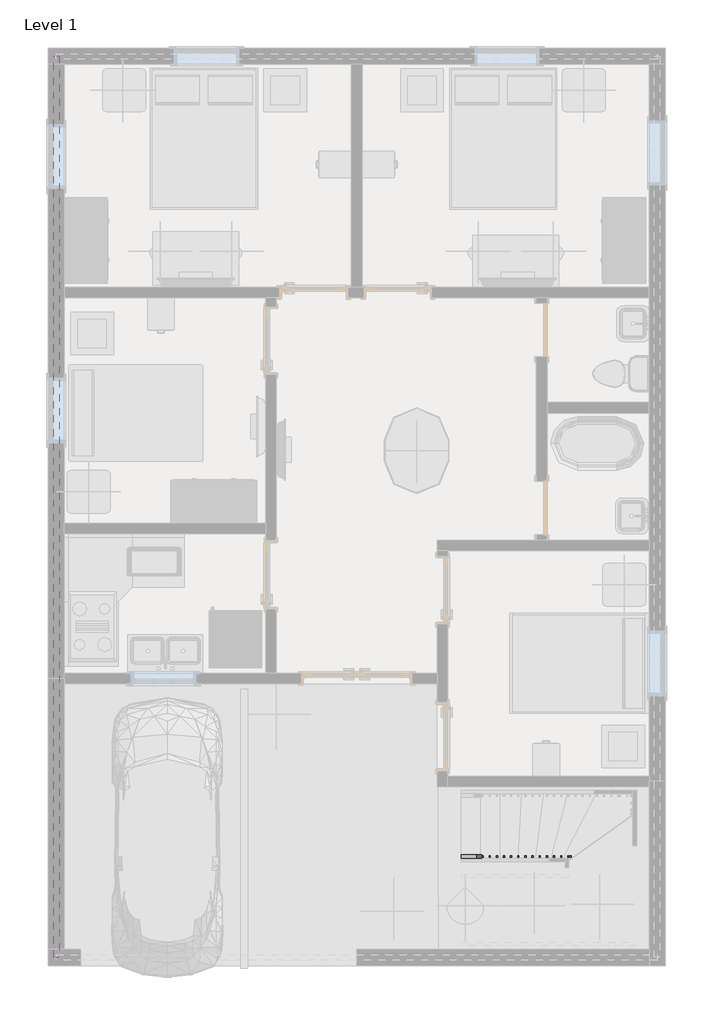
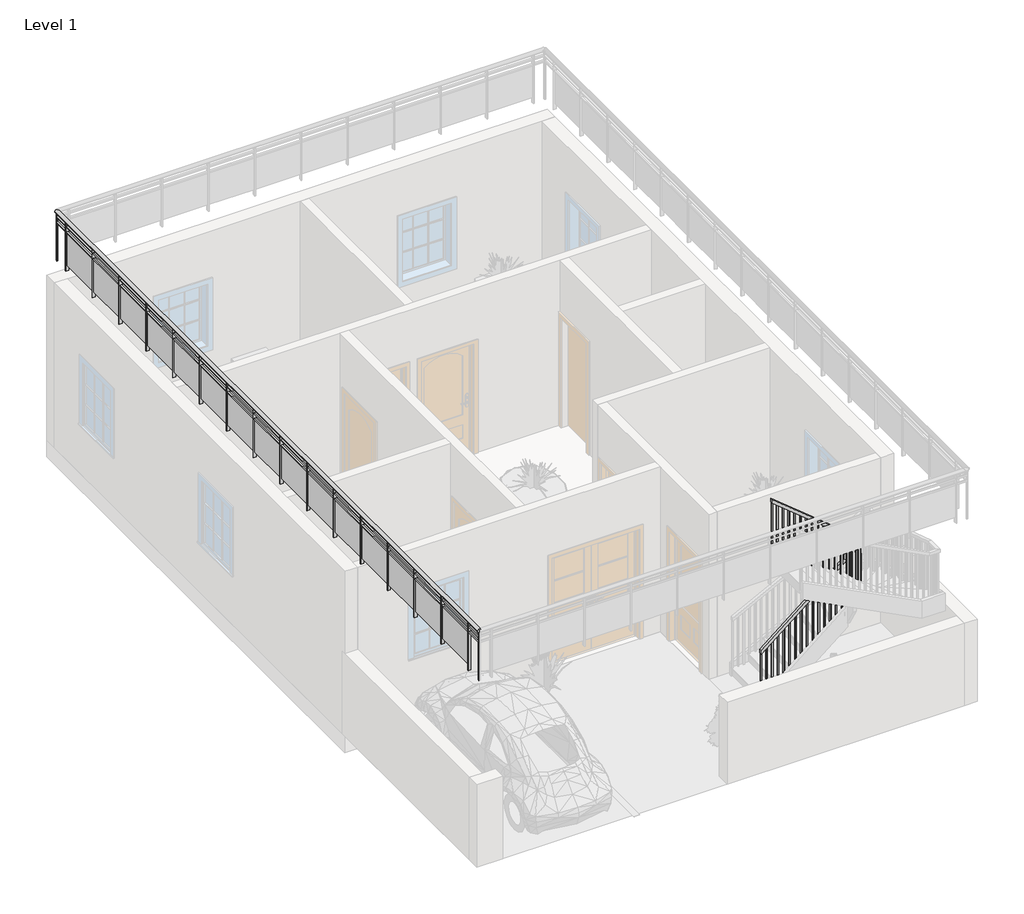
# One storey, part 2 of 4: 2 railings.
"""IFC4 building model written with IfcOpenShell, lengths in millimetres."""

from ifc_helpers import new_model, si_unit, point, frame, origin, place, context, project, spatial, polyline, ellipse_curve, trimmed, outline, extrude, faceted_brep, element, save
from ifc_brep_helpers import plane_surface, extruded_surface, advanced_brep

model = new_model("IFC4")

# Units and contexts
model_context = context("Model", 3, world=origin())
ifc_project = project(units=[si_unit("LENGTHUNIT", "METRE", prefix="MILLI")], contexts=[model_context])

# Site, building, storey
site = spatial("IfcSite", under=ifc_project)
building = spatial("IfcBuilding", under=site)
storey = spatial("IfcBuildingStorey", under=building, Name="Level 1", Elevation=0.0)

# Railings
placement = place(None, origin())
element("IfcRailing", 1, ObjectType="Glass Panel - Bottom Fill", at=placement, inside=storey, context=model_context, shape_type="SolidModel", body=[
    advanced_brep(
    [(-12772.0505662, 285.6645941, 4267.2), (-12695.8505662, 285.6645941, 4267.2), (-12772.0505662, 13087.2645941, 4267.2), (-12695.8505662, 13087.2645941, 4267.2)],
    [
        (0, 1, ellipse_curve(frame((-12733.9505662, 285.6645941, 4267.2), z_axis=(0.0, -1.0, 0.0), x_axis=(1.0, 0.0, 0.0)), 38.1, 28.575)),
        (1, 0, ellipse_curve(frame((-12733.9505662, 285.6645941, 4267.2), z_axis=(0.0, -1.0, 0.0), x_axis=(1.0, 0.0, 0.0)), 38.1, 28.575)),
        (2, 3, ellipse_curve(frame((-12733.9505662, 13087.2645941, 4267.2), z_axis=(0.0, 1.0, 0.0), x_axis=(1.0, 0.0, 0.0)), 38.1, 28.575)),
        (3, 2, ellipse_curve(frame((-12733.9505662, 13087.2645941, 4267.2), z_axis=(0.0, 1.0, 0.0), x_axis=(1.0, 0.0, 0.0)), 38.1, 28.575)),
        (0, 2),
        (3, 1),
    ],
    [
        plane_surface(frame((-12733.9505662, 285.6645941, 4267.2), z_axis=(0.0, -1.0, 0.0), x_axis=(0.0, 0.0, 1.0))),
        plane_surface(frame((-12733.9505662, 13087.2645941, 4267.2), z_axis=(0.0, 1.0, 0.0), x_axis=(0.0, 0.0, 1.0))),
        extruded_surface(trimmed(ellipse_curve(frame((-12733.9505662, 13087.2645941, 4267.2), z_axis=(0.0, -1.0, 0.0), x_axis=(1.0, 0.0, 0.0)), 38.1, 28.575), [point((-12772.0505662, 13087.2645941, 4267.2))], [point((-12695.8505662, 13087.2645941, 4267.2))], True, "CARTESIAN"), (0.0, -12801.599999999999, 0.0), 12801.599999999999),
        extruded_surface(trimmed(ellipse_curve(frame((-12733.9505662, 13087.2645941, 4267.2), z_axis=(0.0, -1.0, 0.0), x_axis=(1.0, 0.0, 0.0)), 38.1, 28.575), [point((-12695.8505662, 13087.2645941, 4267.2))], [point((-12772.0505662, 13087.2645941, 4267.2))], True, "CARTESIAN"), (0.0, -12801.599999999999, 0.0), 12801.599999999999),
    ],
    [
        (0, [[1, 2]]),
        (1, [[3, 4]]),
        (2, [[-1, 5, -4, 6]]),
        (3, [[-2, -6, -3, -5]]),
    ],
),
    extrude(outline(polyline([(-12721.2505662, 285.6645941), (-12746.6505662, 285.6645941), (-12746.6505662, 13087.2645941), (-12721.2505662, 13087.2645941), (-12721.2505662, 285.6645941)])), frame((0.0, 0.0, 4152.9), z_axis=(0.0, 0.0, 1.0), x_axis=(1.0, 0.0, 0.0)), (0.0, 0.0, 1.0), 25.4),
    extrude(outline(polyline([(-12721.2505662, 285.6645941), (-12746.6505662, 285.6645941), (-12746.6505662, 13087.2645941), (-12721.2505662, 13087.2645941), (-12721.2505662, 285.6645941)])), frame((0.0, 0.0, 4051.3), z_axis=(0.0, 0.0, 1.0), x_axis=(1.0, 0.0, 0.0)), (0.0, 0.0, 1.0), 25.4),
    extrude(outline(polyline([(-12708.5505662, 12776.1145941), (-12759.3505662, 12776.1145941), (-12759.3505662, 12788.8145941), (-12708.5505662, 12788.8145941), (-12708.5505662, 12776.1145941)])), frame((0.0, 0.0, 3352.8), z_axis=(0.0, 0.0, 1.0), x_axis=(1.0, 0.0, 0.0)), (0.0, 0.0, 1.0), 885.6788223),
    extrude(outline(polyline([(-12740.4857232, 11969.6645941), (-12740.4857232, 12782.4645941), (-12734.1357232, 12782.4645941), (-12734.1357232, 11969.6645941), (-12740.4857232, 11969.6645941)])), frame((0.0, 0.0, 3454.4), z_axis=(0.0, 0.0, 1.0), x_axis=(1.0, 0.0, 0.0)), (0.0, 0.0, 1.0), 596.9),
    extrude(outline(polyline([(-12708.5505662, 11963.3145941), (-12759.3505662, 11963.3145941), (-12759.3505662, 11976.0145941), (-12708.5505662, 11976.0145941), (-12708.5505662, 11963.3145941)])), frame((0.0, 0.0, 3352.8), z_axis=(0.0, 0.0, 1.0), x_axis=(1.0, 0.0, 0.0)), (0.0, 0.0, 1.0), 885.6788223),
    extrude(outline(polyline([(-12740.4857232, 11156.8645941), (-12740.4857232, 11969.6645941), (-12734.1357232, 11969.6645941), (-12734.1357232, 11156.8645941), (-12740.4857232, 11156.8645941)])), frame((0.0, 0.0, 3454.4), z_axis=(0.0, 0.0, 1.0), x_axis=(1.0, 0.0, 0.0)), (0.0, 0.0, 1.0), 596.9),
    extrude(outline(polyline([(-12708.5505662, 11150.5145941), (-12759.3505662, 11150.5145941), (-12759.3505662, 11163.2145941), (-12708.5505662, 11163.2145941), (-12708.5505662, 11150.5145941)])), frame((0.0, 0.0, 3352.8), z_axis=(0.0, 0.0, 1.0), x_axis=(1.0, 0.0, 0.0)), (0.0, 0.0, 1.0), 885.6788223),
    extrude(outline(polyline([(-12740.4857232, 10344.0645941), (-12740.4857232, 11156.8645941), (-12734.1357232, 11156.8645941), (-12734.1357232, 10344.0645941), (-12740.4857232, 10344.0645941)])), frame((0.0, 0.0, 3454.4), z_axis=(0.0, 0.0, 1.0), x_axis=(1.0, 0.0, 0.0)), (0.0, 0.0, 1.0), 596.9),
    extrude(outline(polyline([(-12708.5505662, 10337.7145941), (-12759.3505662, 10337.7145941), (-12759.3505662, 10350.4145941), (-12708.5505662, 10350.4145941), (-12708.5505662, 10337.7145941)])), frame((0.0, 0.0, 3352.8), z_axis=(0.0, 0.0, 1.0), x_axis=(1.0, 0.0, 0.0)), (0.0, 0.0, 1.0), 885.6788223),
    extrude(outline(polyline([(-12740.4857232, 9531.2645941), (-12740.4857232, 10344.0645941), (-12734.1357232, 10344.0645941), (-12734.1357232, 9531.2645941), (-12740.4857232, 9531.2645941)])), frame((0.0, 0.0, 3454.4), z_axis=(0.0, 0.0, 1.0), x_axis=(1.0, 0.0, 0.0)), (0.0, 0.0, 1.0), 596.9),
    extrude(outline(polyline([(-12708.5505662, 9524.9145941), (-12759.3505662, 9524.9145941), (-12759.3505662, 9537.6145941), (-12708.5505662, 9537.6145941), (-12708.5505662, 9524.9145941)])), frame((0.0, 0.0, 3352.8), z_axis=(0.0, 0.0, 1.0), x_axis=(1.0, 0.0, 0.0)), (0.0, 0.0, 1.0), 885.6788223),
    extrude(outline(polyline([(-12740.4857232, 8718.4645941), (-12740.4857232, 9531.2645941), (-12734.1357232, 9531.2645941), (-12734.1357232, 8718.4645941), (-12740.4857232, 8718.4645941)])), frame((0.0, 0.0, 3454.4), z_axis=(0.0, 0.0, 1.0), x_axis=(1.0, 0.0, 0.0)), (0.0, 0.0, 1.0), 596.9),
    extrude(outline(polyline([(-12708.5505662, 8712.1145941), (-12759.3505662, 8712.1145941), (-12759.3505662, 8724.8145941), (-12708.5505662, 8724.8145941), (-12708.5505662, 8712.1145941)])), frame((0.0, 0.0, 3352.8), z_axis=(0.0, 0.0, 1.0), x_axis=(1.0, 0.0, 0.0)), (0.0, 0.0, 1.0), 885.6788223),
    extrude(outline(polyline([(-12740.4857232, 7905.6645941), (-12740.4857232, 8718.4645941), (-12734.1357232, 8718.4645941), (-12734.1357232, 7905.6645941), (-12740.4857232, 7905.6645941)])), frame((0.0, 0.0, 3454.4), z_axis=(0.0, 0.0, 1.0), x_axis=(1.0, 0.0, 0.0)), (0.0, 0.0, 1.0), 596.9),
    extrude(outline(polyline([(-12708.5505662, 7899.3145941), (-12759.3505662, 7899.3145941), (-12759.3505662, 7912.0145941), (-12708.5505662, 7912.0145941), (-12708.5505662, 7899.3145941)])), frame((0.0, 0.0, 3352.8), z_axis=(0.0, 0.0, 1.0), x_axis=(1.0, 0.0, 0.0)), (0.0, 0.0, 1.0), 885.6788223),
    extrude(outline(polyline([(-12740.4857232, 7092.8645941), (-12740.4857232, 7905.6645941), (-12734.1357232, 7905.6645941), (-12734.1357232, 7092.8645941), (-12740.4857232, 7092.8645941)])), frame((0.0, 0.0, 3454.4), z_axis=(0.0, 0.0, 1.0), x_axis=(1.0, 0.0, 0.0)), (0.0, 0.0, 1.0), 596.9),
    extrude(outline(polyline([(-12708.5505662, 7086.5145941), (-12759.3505662, 7086.5145941), (-12759.3505662, 7099.2145941), (-12708.5505662, 7099.2145941), (-12708.5505662, 7086.5145941)])), frame((0.0, 0.0, 3352.8), z_axis=(0.0, 0.0, 1.0), x_axis=(1.0, 0.0, 0.0)), (0.0, 0.0, 1.0), 885.6788223),
    extrude(outline(polyline([(-12740.4857232, 6280.0645941), (-12740.4857232, 7092.8645941), (-12734.1357232, 7092.8645941), (-12734.1357232, 6280.0645941), (-12740.4857232, 6280.0645941)])), frame((0.0, 0.0, 3454.4), z_axis=(0.0, 0.0, 1.0), x_axis=(1.0, 0.0, 0.0)), (0.0, 0.0, 1.0), 596.9),
    extrude(outline(polyline([(-12708.5505662, 6273.7145941), (-12759.3505662, 6273.7145941), (-12759.3505662, 6286.4145941), (-12708.5505662, 6286.4145941), (-12708.5505662, 6273.7145941)])), frame((0.0, 0.0, 3352.8), z_axis=(0.0, 0.0, 1.0), x_axis=(1.0, 0.0, 0.0)), (0.0, 0.0, 1.0), 885.6788223),
    extrude(outline(polyline([(-12740.4857232, 5467.2645941), (-12740.4857232, 6280.0645941), (-12734.1357232, 6280.0645941), (-12734.1357232, 5467.2645941), (-12740.4857232, 5467.2645941)])), frame((0.0, 0.0, 3454.4), z_axis=(0.0, 0.0, 1.0), x_axis=(1.0, 0.0, 0.0)), (0.0, 0.0, 1.0), 596.9),
    extrude(outline(polyline([(-12708.5505662, 5460.9145941), (-12759.3505662, 5460.9145941), (-12759.3505662, 5473.6145941), (-12708.5505662, 5473.6145941), (-12708.5505662, 5460.9145941)])), frame((0.0, 0.0, 3352.8), z_axis=(0.0, 0.0, 1.0), x_axis=(1.0, 0.0, 0.0)), (0.0, 0.0, 1.0), 885.6788223),
    extrude(outline(polyline([(-12740.4857232, 4654.4645941), (-12740.4857232, 5467.2645941), (-12734.1357232, 5467.2645941), (-12734.1357232, 4654.4645941), (-12740.4857232, 4654.4645941)])), frame((0.0, 0.0, 3454.4), z_axis=(0.0, 0.0, 1.0), x_axis=(1.0, 0.0, 0.0)), (0.0, 0.0, 1.0), 596.9),
    extrude(outline(polyline([(-12708.5505662, 4648.1145941), (-12759.3505662, 4648.1145941), (-12759.3505662, 4660.8145941), (-12708.5505662, 4660.8145941), (-12708.5505662, 4648.1145941)])), frame((0.0, 0.0, 3352.8), z_axis=(0.0, 0.0, 1.0), x_axis=(1.0, 0.0, 0.0)), (0.0, 0.0, 1.0), 885.6788223),
    extrude(outline(polyline([(-12740.4857232, 3841.6645941), (-12740.4857232, 4654.4645941), (-12734.1357232, 4654.4645941), (-12734.1357232, 3841.6645941), (-12740.4857232, 3841.6645941)])), frame((0.0, 0.0, 3454.4), z_axis=(0.0, 0.0, 1.0), x_axis=(1.0, 0.0, 0.0)), (0.0, 0.0, 1.0), 596.9),
    extrude(outline(polyline([(-12708.5505662, 3835.3145941), (-12759.3505662, 3835.3145941), (-12759.3505662, 3848.0145941), (-12708.5505662, 3848.0145941), (-12708.5505662, 3835.3145941)])), frame((0.0, 0.0, 3352.8), z_axis=(0.0, 0.0, 1.0), x_axis=(1.0, 0.0, 0.0)), (0.0, 0.0, 1.0), 885.6788223),
    extrude(outline(polyline([(-12740.4857232, 3028.8645941), (-12740.4857232, 3841.6645941), (-12734.1357232, 3841.6645941), (-12734.1357232, 3028.8645941), (-12740.4857232, 3028.8645941)])), frame((0.0, 0.0, 3454.4), z_axis=(0.0, 0.0, 1.0), x_axis=(1.0, 0.0, 0.0)), (0.0, 0.0, 1.0), 596.9),
    extrude(outline(polyline([(-12708.5505662, 3022.5145941), (-12759.3505662, 3022.5145941), (-12759.3505662, 3035.2145941), (-12708.5505662, 3035.2145941), (-12708.5505662, 3022.5145941)])), frame((0.0, 0.0, 3352.8), z_axis=(0.0, 0.0, 1.0), x_axis=(1.0, 0.0, 0.0)), (0.0, 0.0, 1.0), 885.6788223),
    extrude(outline(polyline([(-12740.4857232, 2216.0645941), (-12740.4857232, 3028.8645941), (-12734.1357232, 3028.8645941), (-12734.1357232, 2216.0645941), (-12740.4857232, 2216.0645941)])), frame((0.0, 0.0, 3454.4), z_axis=(0.0, 0.0, 1.0), x_axis=(1.0, 0.0, 0.0)), (0.0, 0.0, 1.0), 596.9),
    extrude(outline(polyline([(-12708.5505662, 2209.7145941), (-12759.3505662, 2209.7145941), (-12759.3505662, 2222.4145941), (-12708.5505662, 2222.4145941), (-12708.5505662, 2209.7145941)])), frame((0.0, 0.0, 3352.8), z_axis=(0.0, 0.0, 1.0), x_axis=(1.0, 0.0, 0.0)), (0.0, 0.0, 1.0), 885.6788223),
    extrude(outline(polyline([(-12740.4857232, 1403.2645941), (-12740.4857232, 2216.0645941), (-12734.1357232, 2216.0645941), (-12734.1357232, 1403.2645941), (-12740.4857232, 1403.2645941)])), frame((0.0, 0.0, 3454.4), z_axis=(0.0, 0.0, 1.0), x_axis=(1.0, 0.0, 0.0)), (0.0, 0.0, 1.0), 596.9),
    extrude(outline(polyline([(-12708.5505662, 1396.9145941), (-12759.3505662, 1396.9145941), (-12759.3505662, 1409.6145941), (-12708.5505662, 1409.6145941), (-12708.5505662, 1396.9145941)])), frame((0.0, 0.0, 3352.8), z_axis=(0.0, 0.0, 1.0), x_axis=(1.0, 0.0, 0.0)), (0.0, 0.0, 1.0), 885.6788223),
    extrude(outline(polyline([(-12740.4857232, 590.4645941), (-12740.4857232, 1403.2645941), (-12734.1357232, 1403.2645941), (-12734.1357232, 590.4645941), (-12740.4857232, 590.4645941)])), frame((0.0, 0.0, 3454.4), z_axis=(0.0, 0.0, 1.0), x_axis=(1.0, 0.0, 0.0)), (0.0, 0.0, 1.0), 596.9),
    extrude(outline(polyline([(-12708.5505662, 584.1145941), (-12759.3505662, 584.1145941), (-12759.3505662, 596.8145941), (-12708.5505662, 596.8145941), (-12708.5505662, 584.1145941)])), frame((0.0, 0.0, 3352.8), z_axis=(0.0, 0.0, 1.0), x_axis=(1.0, 0.0, 0.0)), (0.0, 0.0, 1.0), 885.6788223),
    extrude(outline(polyline([(-12724.4255662, 13074.5645941), (-12743.4755662, 13074.5645941), (-12743.4755662, 13093.6145941), (-12724.4255662, 13093.6145941), (-12724.4255662, 13074.5645941)])), frame((0.0, 0.0, 3352.8), z_axis=(0.0, 0.0, 1.0), x_axis=(1.0, 0.0, 0.0)), (0.0, 0.0, 1.0), 885.6788223),
    extrude(outline(polyline([(-12724.4255662, 279.3145941), (-12743.4755662, 279.3145941), (-12743.4755662, 298.3645941), (-12724.4255662, 298.3645941), (-12724.4255662, 279.3145941)])), frame((0.0, 0.0, 3352.8), z_axis=(0.0, 0.0, 1.0), x_axis=(1.0, 0.0, 0.0)), (0.0, 0.0, 1.0), 885.6788223),
])
element("IfcRailing", 2, ObjectType="Handrail - Rectangular", at=placement, inside=storey, context=model_context, shape_type="SolidModel", body=[
    faceted_brep([(-6984.582258, 1746.1645941, 1025.2529681), (-6984.582258, 1746.1645941, 959.7067088), (-6984.582258, 1695.3645941, 959.7067088), (-6984.582258, 1695.3645941, 1025.2529681), (-5533.0505662, 1746.1645941, 2208.7848338), (-5482.2505662, 1746.1645941, 2184.659247), (-5482.2505662, 1695.3645941, 2184.659247), (-5533.0505662, 1695.3645941, 2208.7848338), (-5533.0505662, 1746.1645941, 2414.6281882), (-5482.2505662, 1746.1645941, 2363.8281882), (-5482.2505662, 1695.3645941, 2363.8281882), (-5533.0505662, 1695.3645941, 2414.6281882), (-5406.0505662, 1746.1645941, 2414.6281882), (-5406.0505662, 1746.1645941, 2363.8281882), (-5456.8505662, 1695.3645941, 2363.8281882), (-5456.8505662, 1695.3645941, 2414.6281882), (-5406.0505662, 1619.1645941, 2414.6281882), (-5406.0505662, 1590.0432603, 2363.8281882), (-5456.8505662, 1590.0432603, 2363.8281882), (-5456.8505662, 1619.1645941, 2414.6281882), (-5406.0505662, 1492.1645941, 2631.5051451), (-5406.0505662, 1441.3645941, 2617.7256424), (-5456.8505662, 1441.3645941, 2617.7256424), (-5456.8505662, 1492.1645941, 2631.5051451), (-5406.0505662, 1492.1645941, 2837.3484995), (-5406.0505662, 1441.3645941, 2786.5484995), (-5456.8505662, 1441.3645941, 2786.5484995), (-5456.8505662, 1492.1645941, 2837.3484995), (-5406.0505662, 1365.1645941, 2837.3484995), (-5406.0505662, 1365.1645941, 2786.5484995), (-5456.8505662, 1415.9645941, 2786.5484995), (-5456.8505662, 1415.9645941, 2837.3484995), (-5533.0505662, 1365.1645941, 2837.3484995), (-5551.1359793, 1365.1645941, 2786.5484995), (-5551.1359793, 1415.9645941, 2786.5484995), (-5533.0505662, 1415.9645941, 2837.3484995), (-6984.582258, 1365.1645941, 4020.8803652), (-6984.582258, 1415.9645941, 4020.8803652), (-6984.582258, 1415.9645941, 3955.3341059), (-6984.582258, 1365.1645941, 3955.3341059)], [[[0, 1, 2, 3]], [[1, 0, 4, 5]], [[2, 1, 5, 6]], [[3, 2, 6, 7]], [[0, 3, 7, 4]], [[5, 4, 8, 9]], [[6, 5, 9, 10]], [[7, 6, 10, 11]], [[4, 7, 11, 8]], [[9, 8, 12, 13]], [[10, 9, 13, 14]], [[11, 10, 14, 15]], [[8, 11, 15, 12]], [[13, 12, 16, 17]], [[14, 13, 17, 18]], [[15, 14, 18, 19]], [[12, 15, 19, 16]], [[17, 16, 20, 21]], [[18, 17, 21, 22]], [[19, 18, 22, 23]], [[16, 19, 23, 20]], [[21, 20, 24, 25]], [[22, 21, 25, 26]], [[23, 22, 26, 27]], [[20, 23, 27, 24]], [[25, 24, 28, 29]], [[26, 25, 29, 30]], [[27, 26, 30, 31]], [[24, 27, 31, 28]], [[29, 28, 32, 33]], [[30, 29, 33, 34]], [[31, 30, 34, 35]], [[28, 31, 35, 32]], [[36, 37, 38, 39]], [[33, 32, 36, 39]], [[34, 33, 39, 38]], [[35, 34, 38, 37]], [[32, 35, 37, 36]]]),
    extrude(outline(polyline([(3866.2231262, -6875.2929225), (3881.7558784, -6894.3429225), (2878.6666667, -6894.3429225), (2878.6666667, -6875.2929225), (3866.2231262, -6875.2929225)])), frame((0.0, 1381.0395941, 0.0), z_axis=(0.0, 1.0, 0.0), x_axis=(0.0, 0.0, 1.0)), (0.0, 0.0, 1.0), 19.05),
    extrude(outline(polyline([(3783.3817813, -6773.6929225), (3798.9145334, -6792.7429225), (2878.6666667, -6792.7429225), (2878.6666667, -6773.6929225), (3783.3817813, -6773.6929225)])), frame((0.0, 1381.0395941, 0.0), z_axis=(0.0, 1.0, 0.0), x_axis=(0.0, 0.0, 1.0)), (0.0, 0.0, 1.0), 19.05),
    extrude(outline(polyline([(3700.5404364, -6672.0929225), (3716.0731885, -6691.1429225), (2709.3333333, -6691.1429225), (2709.3333333, -6672.0929225), (3700.5404364, -6672.0929225)])), frame((0.0, 1381.0395941, 0.0), z_axis=(0.0, 1.0, 0.0), x_axis=(0.0, 0.0, 1.0)), (0.0, 0.0, 1.0), 19.05),
    extrude(outline(polyline([(3617.6990914, -6570.4929225), (3633.2318436, -6589.5429225), (2709.3333333, -6589.5429225), (2709.3333333, -6570.4929225), (3617.6990914, -6570.4929225)])), frame((0.0, 1381.0395941, 0.0), z_axis=(0.0, 1.0, 0.0), x_axis=(0.0, 0.0, 1.0)), (0.0, 0.0, 1.0), 19.05),
    extrude(outline(polyline([(3534.8577465, -6468.8929225), (3550.3904987, -6487.9429225), (2709.3333333, -6487.9429225), (2709.3333333, -6468.8929225), (3534.8577465, -6468.8929225)])), frame((0.0, 1381.0395941, 0.0), z_axis=(0.0, 1.0, 0.0), x_axis=(0.0, 0.0, 1.0)), (0.0, 0.0, 1.0), 19.05),
    extrude(outline(polyline([(3452.0164016, -6367.2929225), (3467.5491538, -6386.3429225), (2540.0, -6386.3429225), (2540.0, -6367.2929225), (3452.0164016, -6367.2929225)])), frame((0.0, 1381.0395941, 0.0), z_axis=(0.0, 1.0, 0.0), x_axis=(0.0, 0.0, 1.0)), (0.0, 0.0, 1.0), 19.05),
    extrude(outline(polyline([(3369.1750567, -6265.6929225), (3384.7078088, -6284.7429225), (2540.0, -6284.7429225), (2540.0, -6265.6929225), (3369.1750567, -6265.6929225)])), frame((0.0, 1381.0395941, 0.0), z_axis=(0.0, 1.0, 0.0), x_axis=(0.0, 0.0, 1.0)), (0.0, 0.0, 1.0), 19.05),
    extrude(outline(polyline([(3286.3337117, -6164.0929225), (3301.8664639, -6183.1429225), (2540.0, -6183.1429225), (2540.0, -6164.0929225), (3286.3337117, -6164.0929225)])), frame((0.0, 1381.0395941, 0.0), z_axis=(0.0, 1.0, 0.0), x_axis=(0.0, 0.0, 1.0)), (0.0, 0.0, 1.0), 19.05),
    extrude(outline(polyline([(3203.4923668, -6062.4929225), (3219.025119, -6081.5429225), (2370.6666667, -6081.5429225), (2370.6666667, -6062.4929225), (3203.4923668, -6062.4929225)])), frame((0.0, 1381.0395941, 0.0), z_axis=(0.0, 1.0, 0.0), x_axis=(0.0, 0.0, 1.0)), (0.0, 0.0, 1.0), 19.05),
    extrude(outline(polyline([(3120.6510219, -5960.8929225), (3136.1837741, -5979.9429225), (2370.6666667, -5979.9429225), (2370.6666667, -5960.8929225), (3120.6510219, -5960.8929225)])), frame((0.0, 1381.0395941, 0.0), z_axis=(0.0, 1.0, 0.0), x_axis=(0.0, 0.0, 1.0)), (0.0, 0.0, 1.0), 19.05),
    extrude(outline(polyline([(3037.809677, -5859.2929225), (3053.3424291, -5878.3429225), (2201.3333333, -5878.3429225), (2201.3333333, -5859.2929225), (3037.809677, -5859.2929225)])), frame((0.0, 1381.0395941, 0.0), z_axis=(0.0, 1.0, 0.0), x_axis=(0.0, 0.0, 1.0)), (0.0, 0.0, 1.0), 19.05),
    extrude(outline(polyline([(2954.9683321, -5757.6929225), (2970.5010842, -5776.7429225), (2201.3333333, -5776.7429225), (2201.3333333, -5757.6929225), (2954.9683321, -5757.6929225)])), frame((0.0, 1381.0395941, 0.0), z_axis=(0.0, 1.0, 0.0), x_axis=(0.0, 0.0, 1.0)), (0.0, 0.0, 1.0), 19.05),
    extrude(outline(polyline([(2872.1269871, -5656.0929225), (2887.6597393, -5675.1429225), (2032.0, -5675.1429225), (2032.0, -5656.0929225), (2872.1269871, -5656.0929225)])), frame((0.0, 1381.0395941, 0.0), z_axis=(0.0, 1.0, 0.0), x_axis=(0.0, 0.0, 1.0)), (0.0, 0.0, 1.0), 19.05),
    extrude(outline(polyline([(2789.2856422, -5554.4929225), (2804.8183944, -5573.5429225), (2032.0, -5573.5429225), (2032.0, -5554.4929225), (2789.2856422, -5554.4929225)])), frame((0.0, 1381.0395941, 0.0), z_axis=(0.0, 1.0, 0.0), x_axis=(0.0, 0.0, 1.0)), (0.0, 0.0, 1.0), 19.05),
    extrude(outline(polyline([(1493.2536904, 2529.115018), (1512.3036904, 2496.5834745), (1512.3036904, 1524.0), (1493.2536904, 1524.0), (1493.2536904, 2529.115018)])), frame((-5440.9755662, 0.0, 0.0), z_axis=(1.0, 0.0, 0.0), x_axis=(0.0, 1.0, 0.0)), (0.0, 0.0, 1.0), 19.05),
    extrude(outline(polyline([(1594.8536904, 2355.6134525), (1613.9036904, 2323.0819089), (1613.9036904, 1524.0), (1594.8536904, 1524.0), (1594.8536904, 2355.6134525)])), frame((-5440.9755662, 0.0, 0.0), z_axis=(1.0, 0.0, 0.0), x_axis=(0.0, 1.0, 0.0)), (0.0, 0.0, 1.0), 19.05),
    extrude(outline(polyline([(2127.2519138, -5552.657258), (2111.7191617, -5571.707258), (1016.0, -5571.707258), (1016.0, -5552.657258), (2127.2519138, -5552.657258)])), frame((0.0, 1711.2395941, 0.0), z_axis=(0.0, 1.0, 0.0), x_axis=(0.0, 0.0, 1.0)), (0.0, 0.0, 1.0), 19.05),
    extrude(outline(polyline([(2044.4105689, -5654.257258), (2028.8778167, -5673.307258), (1016.0, -5673.307258), (1016.0, -5654.257258), (2044.4105689, -5654.257258)])), frame((0.0, 1711.2395941, 0.0), z_axis=(0.0, 1.0, 0.0), x_axis=(0.0, 0.0, 1.0)), (0.0, 0.0, 1.0), 19.05),
    extrude(outline(polyline([(1961.569224, -5755.857258), (1946.0364718, -5774.907258), (846.6666667, -5774.907258), (846.6666667, -5755.857258), (1961.569224, -5755.857258)])), frame((0.0, 1711.2395941, 0.0), z_axis=(0.0, 1.0, 0.0), x_axis=(0.0, 0.0, 1.0)), (0.0, 0.0, 1.0), 19.05),
    extrude(outline(polyline([(1878.7278791, -5857.457258), (1863.1951269, -5876.507258), (846.6666667, -5876.507258), (846.6666667, -5857.457258), (1878.7278791, -5857.457258)])), frame((0.0, 1711.2395941, 0.0), z_axis=(0.0, 1.0, 0.0), x_axis=(0.0, 0.0, 1.0)), (0.0, 0.0, 1.0), 19.05),
    extrude(outline(polyline([(1795.8865341, -5959.057258), (1780.353782, -5978.107258), (677.3333333, -5978.107258), (677.3333333, -5959.057258), (1795.8865341, -5959.057258)])), frame((0.0, 1711.2395941, 0.0), z_axis=(0.0, 1.0, 0.0), x_axis=(0.0, 0.0, 1.0)), (0.0, 0.0, 1.0), 19.05),
    extrude(outline(polyline([(1713.0451892, -6060.657258), (1697.5124371, -6079.707258), (677.3333333, -6079.707258), (677.3333333, -6060.657258), (1713.0451892, -6060.657258)])), frame((0.0, 1711.2395941, 0.0), z_axis=(0.0, 1.0, 0.0), x_axis=(0.0, 0.0, 1.0)), (0.0, 0.0, 1.0), 19.05),
    extrude(outline(polyline([(1630.2038443, -6162.257258), (1614.6710921, -6181.307258), (508.0, -6181.307258), (508.0, -6162.257258), (1630.2038443, -6162.257258)])), frame((0.0, 1711.2395941, 0.0), z_axis=(0.0, 1.0, 0.0), x_axis=(0.0, 0.0, 1.0)), (0.0, 0.0, 1.0), 19.05),
    extrude(outline(polyline([(1547.3624994, -6263.857258), (1531.8297472, -6282.907258), (508.0, -6282.907258), (508.0, -6263.857258), (1547.3624994, -6263.857258)])), frame((0.0, 1711.2395941, 0.0), z_axis=(0.0, 1.0, 0.0), x_axis=(0.0, 0.0, 1.0)), (0.0, 0.0, 1.0), 19.05),
    extrude(outline(polyline([(1464.5211545, -6365.457258), (1448.9884023, -6384.507258), (508.0, -6384.507258), (508.0, -6365.457258), (1464.5211545, -6365.457258)])), frame((0.0, 1711.2395941, 0.0), z_axis=(0.0, 1.0, 0.0), x_axis=(0.0, 0.0, 1.0)), (0.0, 0.0, 1.0), 19.05),
    extrude(outline(polyline([(1381.6798095, -6467.057258), (1366.1470574, -6486.107258), (338.6666667, -6486.107258), (338.6666667, -6467.057258), (1381.6798095, -6467.057258)])), frame((0.0, 1711.2395941, 0.0), z_axis=(0.0, 1.0, 0.0), x_axis=(0.0, 0.0, 1.0)), (0.0, 0.0, 1.0), 19.05),
    extrude(outline(polyline([(1298.8384646, -6568.657258), (1283.3057124, -6587.707258), (338.6666667, -6587.707258), (338.6666667, -6568.657258), (1298.8384646, -6568.657258)])), frame((0.0, 1711.2395941, 0.0), z_axis=(0.0, 1.0, 0.0), x_axis=(0.0, 0.0, 1.0)), (0.0, 0.0, 1.0), 19.05),
    extrude(outline(polyline([(1215.9971197, -6670.257258), (1200.4643675, -6689.307258), (338.6666667, -6689.307258), (338.6666667, -6670.257258), (1215.9971197, -6670.257258)])), frame((0.0, 1711.2395941, 0.0), z_axis=(0.0, 1.0, 0.0), x_axis=(0.0, 0.0, 1.0)), (0.0, 0.0, 1.0), 19.05),
    extrude(outline(polyline([(1133.1557748, -6771.857258), (1117.6230226, -6790.907258), (169.3333333, -6790.907258), (169.3333333, -6771.857258), (1133.1557748, -6771.857258)])), frame((0.0, 1711.2395941, 0.0), z_axis=(0.0, 1.0, 0.0), x_axis=(0.0, 0.0, 1.0)), (0.0, 0.0, 1.0), 19.05),
    extrude(outline(polyline([(1050.3144298, -6873.457258), (1034.7816777, -6892.507258), (169.3333333, -6892.507258), (169.3333333, -6873.457258), (1050.3144298, -6873.457258)])), frame((0.0, 1711.2395941, 0.0), z_axis=(0.0, 1.0, 0.0), x_axis=(0.0, 0.0, 1.0)), (0.0, 0.0, 1.0), 19.05),
    extrude(outline(polyline([(-5452.8929225, 1400.0895941), (-5452.8929225, 1381.0395941), (-5471.9429225, 1381.0395941), (-5471.9429225, 1400.0895941), (-5452.8929225, 1400.0895941)])), frame((0.0, 0.0, 1862.6666667), z_axis=(0.0, 0.0, 1.0), x_axis=(1.0, 0.0, 0.0)), (0.0, 0.0, 1.0), 923.8818329),
    extrude(outline(polyline([(-5440.9755662, 1400.0895941), (-5421.9255662, 1400.0895941), (-5421.9255662, 1381.0395941), (-5440.9755662, 1381.0395941), (-5440.9755662, 1400.0895941)])), frame((0.0, 0.0, 1862.6666667), z_axis=(0.0, 0.0, 1.0), x_axis=(1.0, 0.0, 0.0)), (0.0, 0.0, 1.0), 923.8818329),
    extrude(outline(polyline([(-5440.9755662, 1414.8754979), (-5421.9255662, 1414.8754979), (-5421.9255662, 1395.8254979), (-5440.9755662, 1395.8254979), (-5440.9755662, 1414.8754979)])), frame((0.0, 0.0, 1693.3333333), z_axis=(0.0, 0.0, 1.0), x_axis=(1.0, 0.0, 0.0)), (0.0, 0.0, 1.0), 1093.2151662),
    extrude(outline(polyline([(-5440.9755662, 1715.5036904), (-5421.9255662, 1715.5036904), (-5421.9255662, 1696.4536904), (-5440.9755662, 1696.4536904), (-5440.9755662, 1715.5036904)])), frame((0.0, 0.0, 1354.6666667), z_axis=(0.0, 0.0, 1.0), x_axis=(1.0, 0.0, 0.0)), (0.0, 0.0, 1.0), 1009.1615215),
    extrude(outline(polyline([(-5440.9755662, 1711.2395941), (-5440.9755662, 1730.2895941), (-5421.9255662, 1730.2895941), (-5421.9255662, 1711.2395941), (-5440.9755662, 1711.2395941)])), frame((0.0, 0.0, 1185.3333333), z_axis=(0.0, 0.0, 1.0), x_axis=(1.0, 0.0, 0.0)), (0.0, 0.0, 1.0), 1178.4948549),
    extrude(outline(polyline([(-5471.9429225, 1711.2395941), (-5471.9429225, 1730.2895941), (-5452.8929225, 1730.2895941), (-5452.8929225, 1711.2395941), (-5471.9429225, 1711.2395941)])), frame((0.0, 0.0, 1185.3333333), z_axis=(0.0, 0.0, 1.0), x_axis=(1.0, 0.0, 0.0)), (0.0, 0.0, 1.0), 1178.4948549),
    extrude(outline(polyline([(3939.8013537, -6965.532258), (3955.3341059, -6984.582258), (2878.6666667, -6984.582258), (2878.6666667, -6965.532258), (3939.8013537, -6965.532258)])), frame((0.0, 1381.0395941, 0.0), z_axis=(0.0, 1.0, 0.0), x_axis=(0.0, 0.0, 1.0)), (0.0, 0.0, 1.0), 19.05),
    extrude(outline(polyline([(975.239461, -6965.532258), (959.7067088, -6984.582258), (169.3333333, -6984.582258), (169.3333333, -6965.532258), (975.239461, -6965.532258)])), frame((0.0, 1711.2395941, 0.0), z_axis=(0.0, 1.0, 0.0), x_axis=(0.0, 0.0, 1.0)), (0.0, 0.0, 1.0), 19.05),
])

save(model, "model.ifc")

# Revit data of these elements
# Type "Glass Panel - Bottom Fill"
#   Assembly Code = "C2010400"
#   built-in parameter 1008612 = 0.0416667 (stored number, unit not read)
#   built-in parameter 1008611 = 0.0416667 (stored number, unit not read)
#   built-in parameter 1008609 = 0.333333 (stored number, unit not read)
#   built-in parameter 1008604 = 0.166667 (stored number, unit not read)
#   built-in parameter 1008603 = 0.166667 (stored number, unit not read)
#   Railing Height = 3' - 0"
#   built-in parameter 1008630 = 2
#   built-in parameter 1008610 = 2
#   built-in parameter 1008618 = Baluster - Square : 3/4"
# Type "Handrail - Rectangular"
#   Assembly Code = "C2010400"
#   built-in parameter 1008612 = 0.0416667 (stored number, unit not read)
#   built-in parameter 1008611 = 0.0416667 (stored number, unit not read)
#   built-in parameter 1008609 = 0.333333 (stored number, unit not read)
#   built-in parameter 1008604 = 0.166667 (stored number, unit not read)
#   built-in parameter 1008603 = 0.166667 (stored number, unit not read)
#   Railing Height = 3' - 0"
#   built-in parameter 1008630 = 2
#   built-in parameter 1008610 = 2
#   built-in parameter 1008618 = Baluster - Square : 3/4"
# Element 1 (IfcRailing, "Glass Panel - Bottom Fill")
#   built-in parameter 1008621 = 11 (stored number, unit not read)
#   Phase Created = New Construction
#   Materials on its faces: "Glass"
# Element 2 (IfcRailing, "Handrail - Rectangular")
#   Phase Created = New Construction
# Materials
#   "Glass": class "Glass", colour RGB 0 128 192, transparency 0.75, Description = "Soda Lime Glass", Cost = 0
